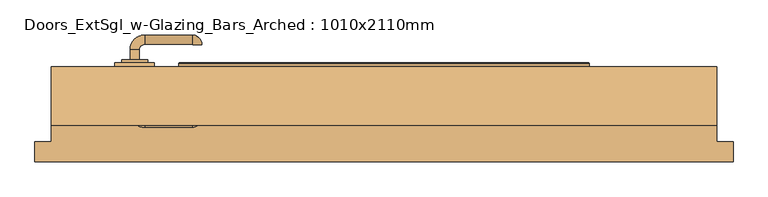
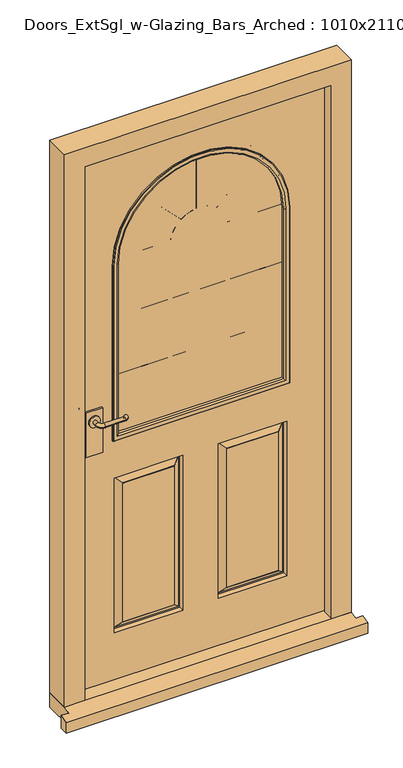
"""IFC4 building model written with IfcOpenShell, lengths in millimetres: door geometry, Doors_ExtSgl_w-Glazing_Bars_Arched : 1010x2110mm."""

from ifc_helpers import new_model, si_unit, point, frame, frame_2d, origin, place, context, project, spatial, polyline, circle_curve, ellipse_curve, trimmed, segment, composite_curve, outline, extrude, faceted_brep, source, transform, mapped, element, save
from ifc_brep_helpers import plane_surface, cylinder_surface, revolved_surface, advanced_brep


def doors_extsgl_w_glazing_bars_arched_1010x2110mm_5c897e1f(model_context):
    return source(origin(), model_context, "Body", "SolidModel", [
        extrude(outline(composite_curve([segment(trimmed(circle_curve(frame_2d((1050.0, -378.5)), 20.0), [point((1050.0, -398.5))], [point((1050.0, -358.5))], False, "CARTESIAN"), True, "CONTINUOUS"), segment(trimmed(circle_curve(frame_2d((1050.0, -378.5)), 20.0), [point((1050.0, -358.5))], [point((1050.0, -398.5))], False, "CARTESIAN"), True, "CONTINUOUS")], self_intersect=False)), frame((0.0, 18.4, 0.0), z_axis=(0.0, 1.0, 0.0), x_axis=(0.0, 0.0, 1.0)), (0.0, 0.0, 1.0), 4.5929895),
        advanced_brep(
        [(-371.5, 22.9929895, 1050.0), (-385.5, 22.9929895, 1050.0), (-371.5, 38.4, 1050.0), (-385.5, 38.4, 1050.0), (-363.5, 60.4, 1050.0), (-363.5, 46.4, 1050.0), (-291.5, 46.4, 1050.0), (-291.5, 60.4, 1050.0), (-290.5, 45.4, 1050.0), (-276.5, 45.4, 1050.0)],
        [
            (0, 1, circle_curve(frame((-378.5, 22.9929895, 1050.0), z_axis=(0.0, -1.0, 0.0), x_axis=(-1.0, 0.0, 0.0)), 7.0)),
            (1, 0, circle_curve(frame((-378.5, 22.9929895, 1050.0), z_axis=(0.0, -1.0, 0.0), x_axis=(-1.0, 0.0, 0.0)), 7.0)),
            (0, 2),
            (2, 3, circle_curve(frame((-378.5, 38.4, 1050.0), z_axis=(0.0, -1.0, 0.0), x_axis=(-1.0, 0.0, 0.0)), 7.0)),
            (3, 1),
            (3, 2, circle_curve(frame((-378.5, 38.4, 1050.0), z_axis=(0.0, -1.0, 0.0), x_axis=(-1.0, 0.0, 0.0)), 7.0)),
            (4, 3, circle_curve(frame((-363.5, 38.4, 1050.0), z_axis=(0.0, 0.0, 1.0), x_axis=(-1.0, 0.0, 0.0)), 22.0)),
            (2, 5, circle_curve(frame((-363.5, 38.4, 1050.0), z_axis=(0.0, 0.0, -1.0), x_axis=(-1.0, 0.0, 0.0)), 8.0)),
            (5, 4, circle_curve(frame((-363.5, 53.4, 1050.0), z_axis=(-1.0, 0.0, 0.0), x_axis=(0.0, 1.0, 0.0)), 7.0)),
            (4, 5, circle_curve(frame((-363.5, 53.4, 1050.0), z_axis=(-1.0, 0.0, 0.0), x_axis=(0.0, 1.0, 0.0)), 7.0)),
            (5, 6),
            (6, 7, circle_curve(frame((-291.5, 53.4, 1050.0), z_axis=(-1.0, 0.0, 0.0), x_axis=(0.0, 1.0, 0.0)), 7.0)),
            (7, 4),
            (7, 6, circle_curve(frame((-291.5, 53.4, 1050.0), z_axis=(-1.0, 0.0, 0.0), x_axis=(0.0, 1.0, 0.0)), 7.0)),
            (8, 9, circle_curve(frame((-283.5, 45.4, 1050.0), z_axis=(0.0, -1.0, 0.0), x_axis=(1.0, 0.0, 0.0)), 7.0)),
            (9, 8, circle_curve(frame((-283.5, 45.4, 1050.0), z_axis=(0.0, -1.0, 0.0), x_axis=(1.0, 0.0, 0.0)), 7.0)),
            (9, 7, circle_curve(frame((-291.5, 45.4, 1050.0), z_axis=(0.0, 0.0, 1.0), x_axis=(0.0, 1.0, 0.0)), 15.0)),
            (6, 8, circle_curve(frame((-291.5, 45.4, 1050.0), z_axis=(0.0, 0.0, -1.0), x_axis=(0.0, 1.0, 0.0)), 1.0)),
        ],
        [
            plane_surface(frame((-378.5, 22.9929895, 1050.0), z_axis=(0.0, -1.0, 0.0), x_axis=(0.0, 0.0, 1.0))),
            cylinder_surface(frame((-378.5, 22.9929895, 1050.0), z_axis=(0.0, -1.0, 0.0), x_axis=(-1.0, 0.0, 0.0)), 7.0),
            revolved_surface(trimmed(ellipse_curve(frame((-378.5, 38.4, 1050.0), z_axis=(0.0, -1.0, 0.0), x_axis=(-1.0, 0.0, 0.0)), 7.0, 7.0), [point((-371.5, 38.4, 1050.0))], [point((-385.5, 38.4, 1050.0))], True, "CARTESIAN"), (-363.5, 38.4, 1050.0), (0.0, 0.0, -1.0)),
            revolved_surface(trimmed(ellipse_curve(frame((-378.5, 38.4, 1050.0), z_axis=(0.0, -1.0, 0.0), x_axis=(-1.0, 0.0, 0.0)), 7.0, 7.0), [point((-385.5, 38.4, 1050.0))], [point((-371.5, 38.4, 1050.0))], True, "CARTESIAN"), (-363.5, 38.4, 1050.0), (0.0, 0.0, -1.0)),
            cylinder_surface(frame((-363.5, 53.4, 1050.0), z_axis=(-1.0, 0.0, 0.0), x_axis=(0.0, 1.0, 0.0)), 7.0),
            plane_surface(frame((-283.5, 45.4, 1050.0), z_axis=(0.0, -1.0, 0.0), x_axis=(0.0, 0.0, 1.0))),
            revolved_surface(trimmed(ellipse_curve(frame((-291.5, 53.4, 1050.0), z_axis=(-1.0, 0.0, 0.0), x_axis=(0.0, 1.0, 0.0)), 7.0, 7.0), [point((-291.5, 46.4, 1050.0))], [point((-291.5, 60.4, 1050.0))], True, "CARTESIAN"), (-291.5, 45.4, 1050.0), (0.0, 0.0, -1.0)),
            revolved_surface(trimmed(ellipse_curve(frame((-291.5, 53.4, 1050.0), z_axis=(-1.0, 0.0, 0.0), x_axis=(0.0, 1.0, 0.0)), 7.0, 7.0), [point((-291.5, 60.4, 1050.0))], [point((-291.5, 46.4, 1050.0))], True, "CARTESIAN"), (-291.5, 45.4, 1050.0), (0.0, 0.0, -1.0)),
        ],
        [
            (0, [[1, 2]]),
            (1, [[-1, 3, 4, 5]]),
            (1, [[-2, -5, 6, -3]]),
            (2, [[7, -4, 8, 9]]),
            (3, [[-8, -6, -7, 10]]),
            (4, [[-9, 11, 12, 13]]),
            (4, [[-10, -13, 14, -11]]),
            (5, [[15, 16]]),
            (6, [[17, -12, 18, -16]]),
            (7, [[-18, -14, -17, -15]]),
        ],
    ),
        extrude(outline(polyline([(-348.5, 12.4), (-408.5, 12.4), (-408.5, 18.4), (-348.5, 18.4), (-348.5, 12.4)])), frame((0.0, 0.0, 925.0), z_axis=(0.0, 0.0, 1.0), x_axis=(1.0, 0.0, 0.0)), (0.0, 0.0, 1.0), 165.0),
        extrude(outline(composite_curve([segment(trimmed(circle_curve(frame_2d((1050.0, -378.5)), 20.0), [point((1050.0, -398.5))], [point((1050.0, -358.5))], False, "CARTESIAN"), True, "CONTINUOUS"), segment(trimmed(circle_curve(frame_2d((1050.0, -378.5)), 20.0), [point((1050.0, -358.5))], [point((1050.0, -398.5))], False, "CARTESIAN"), True, "CONTINUOUS")], self_intersect=False)), frame((0.0, -42.1929895, 0.0), z_axis=(0.0, 1.0, 0.0), x_axis=(0.0, 0.0, 1.0)), (0.0, 0.0, 1.0), 4.5929895),
        advanced_brep(
        [(-371.5, -42.1929895, 1050.0), (-385.5, -42.1929895, 1050.0), (-385.5, -57.6, 1050.0), (-371.5, -57.6, 1050.0), (-363.5, -79.6, 1050.0), (-363.5, -65.6, 1050.0), (-291.5, -79.6, 1050.0), (-291.5, -65.6, 1050.0), (-290.5, -64.6, 1050.0), (-276.5, -64.6, 1050.0)],
        [
            (0, 1, circle_curve(frame((-378.5, -42.1929895, 1050.0), z_axis=(0.0, 1.0, 0.0), x_axis=(-1.0, 0.0, 0.0)), 7.0)),
            (1, 0, circle_curve(frame((-378.5, -42.1929895, 1050.0), z_axis=(0.0, 1.0, 0.0), x_axis=(-1.0, 0.0, 0.0)), 7.0)),
            (1, 2),
            (2, 3, circle_curve(frame((-378.5, -57.6, 1050.0), z_axis=(0.0, 1.0, 0.0), x_axis=(-1.0, 0.0, 0.0)), 7.0)),
            (3, 0),
            (3, 2, circle_curve(frame((-378.5, -57.6, 1050.0), z_axis=(0.0, 1.0, 0.0), x_axis=(-1.0, 0.0, 0.0)), 7.0)),
            (4, 5, circle_curve(frame((-363.5, -72.6, 1050.0), z_axis=(-1.0, 0.0, 0.0), x_axis=(0.0, -1.0, 0.0)), 7.0)),
            (5, 3, circle_curve(frame((-363.5, -57.6, 1050.0), z_axis=(0.0, 0.0, -1.0), x_axis=(-1.0, 0.0, 0.0)), 8.0)),
            (2, 4, circle_curve(frame((-363.5, -57.6, 1050.0), z_axis=(0.0, 0.0, 1.0), x_axis=(-1.0, 0.0, 0.0)), 22.0)),
            (5, 4, circle_curve(frame((-363.5, -72.6, 1050.0), z_axis=(-1.0, 0.0, 0.0), x_axis=(0.0, -1.0, 0.0)), 7.0)),
            (4, 6),
            (6, 7, circle_curve(frame((-291.5, -72.6, 1050.0), z_axis=(-1.0, 0.0, 0.0), x_axis=(0.0, -1.0, 0.0)), 7.0)),
            (7, 5),
            (7, 6, circle_curve(frame((-291.5, -72.6, 1050.0), z_axis=(-1.0, 0.0, 0.0), x_axis=(0.0, -1.0, 0.0)), 7.0)),
            (8, 9, circle_curve(frame((-283.5, -64.6, 1050.0), z_axis=(0.0, 1.0, 0.0), x_axis=(1.0, 0.0, 0.0)), 7.0)),
            (9, 8, circle_curve(frame((-283.5, -64.6, 1050.0), z_axis=(0.0, 1.0, 0.0), x_axis=(1.0, 0.0, 0.0)), 7.0)),
            (8, 7, circle_curve(frame((-291.5, -64.6, 1050.0), z_axis=(0.0, 0.0, -1.0), x_axis=(0.0, -1.0, 0.0)), 1.0)),
            (6, 9, circle_curve(frame((-291.5, -64.6, 1050.0), z_axis=(0.0, 0.0, 1.0), x_axis=(0.0, -1.0, 0.0)), 15.0)),
        ],
        [
            plane_surface(frame((-378.5, -42.1929895, 1050.0), z_axis=(0.0, 1.0, 0.0), x_axis=(0.0, 0.0, 1.0))),
            cylinder_surface(frame((-378.5, -42.1929895, 1050.0), z_axis=(0.0, 1.0, 0.0), x_axis=(-1.0, 0.0, 0.0)), 7.0),
            revolved_surface(trimmed(ellipse_curve(frame((-378.5, -57.6, 1050.0), z_axis=(0.0, -1.0, 0.0), x_axis=(-1.0, 0.0, 0.0)), 7.0, 7.0), [point((-371.5, -57.6, 1050.0))], [point((-385.5, -57.6, 1050.0))], True, "CARTESIAN"), (-363.5, -57.6, 1050.0), (0.0, 0.0, -1.0)),
            revolved_surface(trimmed(ellipse_curve(frame((-378.5, -57.6, 1050.0), z_axis=(0.0, -1.0, 0.0), x_axis=(-1.0, 0.0, 0.0)), 7.0, 7.0), [point((-385.5, -57.6, 1050.0))], [point((-371.5, -57.6, 1050.0))], True, "CARTESIAN"), (-363.5, -57.6, 1050.0), (0.0, 0.0, -1.0)),
            cylinder_surface(frame((-363.5, -72.6, 1050.0), z_axis=(-1.0, 0.0, 0.0), x_axis=(0.0, -1.0, 0.0)), 7.0),
            plane_surface(frame((-283.5, -64.6, 1050.0), z_axis=(0.0, 1.0, 0.0), x_axis=(0.0, 0.0, 1.0))),
            revolved_surface(trimmed(ellipse_curve(frame((-291.5, -72.6, 1050.0), z_axis=(1.0, 0.0, 0.0), x_axis=(0.0, -1.0, 0.0)), 7.0, 7.0), [point((-291.5, -65.6, 1050.0))], [point((-291.5, -79.6, 1050.0))], True, "CARTESIAN"), (-291.5, -64.6, 1050.0), (0.0, 0.0, -1.0)),
            revolved_surface(trimmed(ellipse_curve(frame((-291.5, -72.6, 1050.0), z_axis=(1.0, 0.0, 0.0), x_axis=(0.0, -1.0, 0.0)), 7.0, 7.0), [point((-291.5, -79.6, 1050.0))], [point((-291.5, -65.6, 1050.0))], True, "CARTESIAN"), (-291.5, -64.6, 1050.0), (0.0, 0.0, -1.0)),
        ],
        [
            (0, [[1, 2]]),
            (1, [[3, 4, 5, -2]]),
            (1, [[-5, 6, -3, -1]]),
            (2, [[7, 8, -4, 9]]),
            (3, [[10, -9, -6, -8]]),
            (4, [[11, 12, 13, -7]]),
            (4, [[-13, 14, -11, -10]]),
            (5, [[15, 16]]),
            (6, [[-15, 17, -12, 18]]),
            (7, [[-16, -18, -14, -17]]),
        ],
    ),
        extrude(outline(polyline([(-348.5, -31.6), (-348.5, -37.6), (-408.5, -37.6), (-408.5, -31.6), (-348.5, -31.6)])), frame((0.0, 0.0, 925.0), z_axis=(0.0, 0.0, 1.0), x_axis=(1.0, 0.0, 0.0)), (0.0, 0.0, 1.0), 165.0),
        faceted_brep([(434.5, -76.6, 54.5), (434.5, -34.6, 54.5), (456.5, -34.6, 54.5), (456.5, 12.4, 54.5), (505.0, 12.4, 54.5), (505.0, -76.6, 54.5), (505.0, -76.6, 2110.0), (-505.0, -76.6, 2110.0), (-505.0, -76.6, 54.5), (-434.5, -76.6, 54.5), (-434.5, -76.6, 2039.5), (434.5, -76.6, 2039.5), (505.0, 12.4, 2110.0), (456.5, 12.4, 2061.5), (-456.5, 12.4, 2061.5), (-456.5, 12.4, 54.5), (-505.0, 12.4, 54.5), (-505.0, 12.4, 2110.0), (456.5, -34.6, 2061.5), (434.5, -34.6, 2039.5), (-434.5, -34.6, 2039.5), (-434.5, -34.6, 54.5), (-456.5, -34.6, 54.5), (-456.5, -34.6, 2061.5)], [[[0, 1, 2, 3, 4, 5]], [[5, 6, 7, 8, 9, 10, 11, 0]], [[4, 12, 6, 5]], [[3, 13, 14, 15, 16, 17, 12, 4]], [[2, 18, 13, 3]], [[1, 19, 20, 21, 22, 23, 18, 2]], [[0, 11, 19, 1]], [[9, 21, 20, 10]], [[8, 16, 15, 22, 21, 9]], [[7, 17, 16, 8]], [[14, 23, 22, 15]], [[6, 12, 17, 7]], [[13, 18, 23, 14]], [[10, 20, 19, 11]]]),
        advanced_brep(
        [(453.5, 12.4, 58.5), (-454.4250294, 12.4, 58.5), (-454.4250294, 12.4, 2058.5), (453.5, 12.4, 2058.5), (-303.5, 12.4, 958.5), (303.5, 12.4, 958.5), (303.5, 12.4, 1605.0), (-303.5, 12.4, 1605.0), (-62.5, 12.4, 808.5), (-303.5, 12.4, 808.5), (-303.5, 12.4, 233.5), (-62.5, 12.4, 233.5), (303.5, 12.4, 808.5), (62.5, 12.4, 808.5), (62.5, 12.4, 233.5), (303.5, 12.4, 233.5), (-92.5, 12.4, 263.5), (-273.5, 12.4, 263.5), (-273.5, 12.4, 778.5), (-92.5, 12.4, 778.5), (273.5, 12.4, 263.5), (92.5, 12.4, 263.5), (92.5, 12.4, 778.5), (273.5, 12.4, 778.5), (453.5, -31.6, 58.5), (453.5, -31.6, 2058.5), (-454.4250294, -31.6, 2058.5), (-454.4250294, -31.6, 58.5), (-303.5, -31.6, 958.5), (-303.5, -31.6, 1605.0), (303.5, -31.6, 1605.0), (303.5, -31.6, 958.5), (62.5, -31.6, 808.5), (303.5, -31.6, 808.5), (303.5, -31.6, 233.5), (62.5, -31.6, 233.5), (-303.5, -31.6, 808.5), (-62.5, -31.6, 808.5), (-62.5, -31.6, 233.5), (-303.5, -31.6, 233.5), (92.5, -31.6, 263.5), (273.5, -31.6, 263.5), (273.5, -31.6, 778.5), (92.5, -31.6, 778.5), (-273.5, -31.6, 263.5), (-92.5, -31.6, 263.5), (-92.5, -31.6, 778.5), (-273.5, -31.6, 778.5), (65.5, -16.6, 805.5), (65.5, -16.6, 236.5), (90.5, -30.6, 780.5), (70.5, -16.6, 800.5), (70.5, -16.6, 241.5), (90.5, -30.6, 261.5), (92.5, -30.6, 778.5), (92.5, -30.6, 263.5), (300.5, -16.6, 236.5), (295.5, -16.6, 241.5), (275.5, -30.6, 261.5), (273.5, -30.6, 263.5), (300.5, -16.6, 805.5), (295.5, -16.6, 800.5), (275.5, -30.6, 780.5), (273.5, -30.6, 778.5), (-300.5, -16.6, 805.5), (-300.5, -16.6, 236.5), (-275.5, -30.6, 780.5), (-295.5, -16.6, 800.5), (-295.5, -16.6, 241.5), (-275.5, -30.6, 261.5), (-273.5, -30.6, 778.5), (-273.5, -30.6, 263.5), (-65.5, -16.6, 236.5), (-70.5, -16.6, 241.5), (-90.5, -30.6, 261.5), (-92.5, -30.6, 263.5), (-65.5, -16.6, 805.5), (-70.5, -16.6, 800.5), (-90.5, -30.6, 780.5), (-92.5, -30.6, 778.5), (-92.5, 11.4, 263.5), (-92.5, 11.4, 778.5), (-70.5, -2.6, 241.5), (-90.5, 11.4, 261.5), (-90.5, 11.4, 780.5), (-70.5, -2.6, 800.5), (-65.5, -2.6, 236.5), (-65.5, -2.6, 805.5), (-273.5, 11.4, 778.5), (-275.5, 11.4, 780.5), (-295.5, -2.6, 800.5), (-300.5, -2.6, 805.5), (-273.5, 11.4, 263.5), (-275.5, 11.4, 261.5), (-295.5, -2.6, 241.5), (-300.5, -2.6, 236.5), (300.5, -2.6, 805.5), (300.5, -2.6, 236.5), (275.5, 11.4, 780.5), (295.5, -2.6, 800.5), (295.5, -2.6, 241.5), (275.5, 11.4, 261.5), (273.5, 11.4, 778.5), (273.5, 11.4, 263.5), (65.5, -2.6, 236.5), (70.5, -2.6, 241.5), (90.5, 11.4, 261.5), (92.5, 11.4, 263.5), (65.5, -2.6, 805.5), (70.5, -2.6, 800.5), (90.5, 11.4, 780.5), (92.5, 11.4, 778.5)],
        [
            (0, 1),
            (1, 2),
            (2, 3),
            (3, 0),
            (4, 5),
            (5, 6),
            (6, 7, circle_curve(frame((0.0, 12.4, 1605.0), z_axis=(0.0, -1.0, 0.0), x_axis=(1.0, 0.0, 0.0)), 303.5)),
            (7, 4),
            (8, 9),
            (9, 10),
            (10, 11),
            (11, 8),
            (12, 13),
            (13, 14),
            (14, 15),
            (15, 12),
            (16, 17),
            (17, 18),
            (18, 19),
            (19, 16),
            (20, 21),
            (21, 22),
            (22, 23),
            (23, 20),
            (24, 25),
            (25, 26),
            (26, 27),
            (27, 24),
            (28, 29),
            (29, 30, circle_curve(frame((0.0, -31.6, 1605.0), z_axis=(0.0, 1.0, 0.0), x_axis=(1.0, 0.0, 0.0)), 303.5)),
            (30, 31),
            (31, 28),
            (32, 33),
            (33, 34),
            (34, 35),
            (35, 32),
            (36, 37),
            (37, 38),
            (38, 39),
            (39, 36),
            (40, 41),
            (41, 42),
            (42, 43),
            (43, 40),
            (44, 45),
            (45, 46),
            (46, 47),
            (47, 44),
            (3, 25),
            (24, 0),
            (2, 26),
            (1, 27),
            (7, 29),
            (28, 4),
            (6, 30),
            (5, 31),
            (48, 32),
            (35, 49),
            (49, 48),
            (50, 51),
            (51, 52),
            (52, 53),
            (53, 50),
            (43, 54),
            (54, 55),
            (55, 40),
            (34, 56),
            (56, 49),
            (52, 57),
            (57, 58),
            (58, 53),
            (55, 59),
            (59, 41),
            (33, 60),
            (60, 56),
            (57, 61),
            (61, 62),
            (62, 58),
            (59, 63),
            (63, 42),
            (48, 60),
            (51, 61),
            (50, 62),
            (54, 63),
            (64, 36),
            (39, 65),
            (65, 64),
            (66, 67),
            (67, 68),
            (68, 69),
            (69, 66),
            (47, 70),
            (70, 71),
            (71, 44),
            (38, 72),
            (72, 65),
            (68, 73),
            (73, 74),
            (74, 69),
            (71, 75),
            (75, 45),
            (37, 76),
            (76, 72),
            (73, 77),
            (77, 78),
            (78, 74),
            (75, 79),
            (79, 46),
            (64, 76),
            (67, 77),
            (66, 78),
            (70, 79),
            (80, 16),
            (19, 81),
            (81, 80),
            (82, 83),
            (83, 84),
            (84, 85),
            (85, 82),
            (11, 86),
            (86, 87),
            (87, 8),
            (18, 88),
            (88, 81),
            (84, 89),
            (89, 90),
            (90, 85),
            (87, 91),
            (91, 9),
            (17, 92),
            (92, 88),
            (89, 93),
            (93, 94),
            (94, 90),
            (91, 95),
            (95, 10),
            (80, 92),
            (83, 93),
            (82, 94),
            (86, 95),
            (96, 12),
            (15, 97),
            (97, 96),
            (98, 99),
            (99, 100),
            (100, 101),
            (101, 98),
            (23, 102),
            (102, 103),
            (103, 20),
            (14, 104),
            (104, 97),
            (100, 105),
            (105, 106),
            (106, 101),
            (103, 107),
            (107, 21),
            (13, 108),
            (108, 104),
            (105, 109),
            (109, 110),
            (110, 106),
            (107, 111),
            (111, 22),
            (96, 108),
            (99, 109),
            (98, 110),
            (102, 111),
        ],
        [
            plane_surface(frame((453.5, 12.4, 58.5), z_axis=(0.0, 1.0, 0.0), x_axis=(0.0, 0.0, 1.0))),
            plane_surface(frame((453.5, -31.6, 58.5), z_axis=(0.0, -1.0, 0.0), x_axis=(0.0, 0.0, -1.0))),
            plane_surface(frame((453.5, 12.4, 58.5), z_axis=(1.0, 0.0, 0.0), x_axis=(0.0, -1.0, 0.0))),
            plane_surface(frame((453.5, 12.4, 2058.5), z_axis=(0.0, 0.0, 1.0), x_axis=(0.0, -1.0, 0.0))),
            plane_surface(frame((-454.4250294, 12.4, 2058.5), z_axis=(-1.0, 0.0, 0.0), x_axis=(0.0, -1.0, 0.0))),
            plane_surface(frame((-454.4250294, 12.4, 58.5), z_axis=(0.0, 0.0, -1.0), x_axis=(0.0, -1.0, 0.0))),
            plane_surface(frame((-303.5, 12.4, 958.5), z_axis=(1.0, 0.0, 0.0), x_axis=(0.0, -1.0, 0.0))),
            revolved_surface(polyline([(303.5, -31.6, 1605.0), (303.5, 12.4, 1605.0)]), (0.0, 12.4, 1605.0), (0.0, -1.0, 0.0)),
            plane_surface(frame((303.5, 12.4, 1605.0), z_axis=(-1.0, 0.0, 0.0), x_axis=(0.0, -1.0, 0.0))),
            plane_surface(frame((303.5, 12.4, 958.5), z_axis=(0.0, 0.0, 1.0), x_axis=(0.0, -1.0, 0.0))),
            plane_surface(frame((62.5, -31.6, 808.5), z_axis=(0.9805806756909202, -0.19611613513818407, 0.0), x_axis=(0.0, 0.0, -1.0))),
            plane_surface(frame((70.5, -16.6, 800.5), z_axis=(-0.5734623443633278, -0.8192319205190408, 0.0), x_axis=(0.0, 0.0, -1.0))),
            plane_surface(frame((92.5, -30.6, 778.5), z_axis=(-1.0, 0.0, 0.0), x_axis=(0.0, 0.0, -1.0))),
            plane_surface(frame((62.5, -31.6, 233.5), z_axis=(0.0, -0.19611613513818726, 0.9805806756909196), x_axis=(1.0, 0.0, 0.0))),
            plane_surface(frame((70.5, -16.6, 241.5), z_axis=(0.0, -0.819231920519039, -0.5734623443633305), x_axis=(1.0, 0.0, 0.0))),
            plane_surface(frame((92.5, -30.6, 263.5), z_axis=(0.0, 0.0, -1.0), x_axis=(1.0, 0.0, 0.0))),
            plane_surface(frame((303.5, -31.6, 233.5), z_axis=(-0.9805806756909189, -0.19611613513819046, 0.0), x_axis=(0.0, 0.0, 1.0))),
            plane_surface(frame((295.5, -16.6, 241.5), z_axis=(0.5734623443633332, -0.8192319205190371, 0.0), x_axis=(0.0, 0.0, 1.0))),
            plane_surface(frame((273.5, -30.6, 263.5), z_axis=(1.0, 0.0, 0.0), x_axis=(0.0, 0.0, 1.0))),
            plane_surface(frame((303.5, -31.6, 808.5), z_axis=(0.0, -0.19611613513818726, -0.9805806756909196), x_axis=(-1.0, 0.0, 0.0))),
            plane_surface(frame((300.5, -16.6, 805.5), z_axis=(0.0, -1.0, 0.0), x_axis=(-1.0, 0.0, 0.0))),
            plane_surface(frame((295.5, -16.6, 800.5), z_axis=(0.0, -0.819231920519039, 0.5734623443633305), x_axis=(-1.0, 0.0, 0.0))),
            plane_surface(frame((275.5, -30.6, 780.5), z_axis=(0.0, -1.0, 0.0), x_axis=(-1.0, 0.0, 0.0))),
            plane_surface(frame((273.5, -30.6, 778.5), z_axis=(0.0, 0.0, 1.0), x_axis=(-1.0, 0.0, 0.0))),
            plane_surface(frame((-303.5, -31.6, 808.5), z_axis=(0.9805806756909202, -0.19611613513818407, 0.0), x_axis=(0.0, 0.0, -1.0))),
            plane_surface(frame((-295.5, -16.6, 800.5), z_axis=(-0.5734623443633278, -0.8192319205190408, 0.0), x_axis=(0.0, 0.0, -1.0))),
            plane_surface(frame((-273.5, -30.6, 778.5), z_axis=(-1.0, 0.0, 0.0), x_axis=(0.0, 0.0, -1.0))),
            plane_surface(frame((-303.5, -31.6, 233.5), z_axis=(0.0, -0.19611613513818724, 0.9805806756909196), x_axis=(1.0, 0.0, 0.0))),
            plane_surface(frame((-295.5, -16.6, 241.5), z_axis=(0.0, -0.819231920519039, -0.5734623443633305), x_axis=(1.0, 0.0, 0.0))),
            plane_surface(frame((-273.5, -30.6, 263.5), z_axis=(0.0, 0.0, -1.0), x_axis=(1.0, 0.0, 0.0))),
            plane_surface(frame((-62.5, -31.6, 233.5), z_axis=(-0.9805806756909189, -0.1961161351381904, 0.0), x_axis=(0.0, 0.0, 1.0))),
            plane_surface(frame((-70.5, -16.6, 241.5), z_axis=(0.5734623443633332, -0.8192319205190371, 0.0), x_axis=(0.0, 0.0, 1.0))),
            plane_surface(frame((-92.5, -30.6, 263.5), z_axis=(1.0, 0.0, 0.0), x_axis=(0.0, 0.0, 1.0))),
            plane_surface(frame((-62.5, -31.6, 808.5), z_axis=(0.0, -0.19611613513818724, -0.9805806756909196), x_axis=(-1.0, 0.0, 0.0))),
            plane_surface(frame((-65.5, -16.6, 805.5), z_axis=(0.0, -1.0, 0.0), x_axis=(-1.0, 0.0, 0.0))),
            plane_surface(frame((-70.5, -16.6, 800.5), z_axis=(0.0, -0.819231920519039, 0.5734623443633305), x_axis=(-1.0, 0.0, 0.0))),
            plane_surface(frame((-90.5, -30.6, 780.5), z_axis=(0.0, -1.0, 0.0), x_axis=(-1.0, 0.0, 0.0))),
            plane_surface(frame((-92.5, -30.6, 778.5), z_axis=(0.0, 0.0, 1.0), x_axis=(-1.0, 0.0, 0.0))),
            plane_surface(frame((-92.5, 12.4, 263.5), z_axis=(1.0, 0.0, 0.0), x_axis=(0.0, 0.0, 1.0))),
            plane_surface(frame((-90.5, 11.4, 261.5), z_axis=(0.5734623443633224, 0.8192319205190447, 0.0), x_axis=(0.0, 0.0, 1.0))),
            plane_surface(frame((-65.5, -2.6, 236.5), z_axis=(-0.9805806756909214, 0.1961161351381778, 0.0), x_axis=(0.0, 0.0, 1.0))),
            plane_surface(frame((-92.5, 12.4, 778.5), z_axis=(0.0, 0.0, 1.0), x_axis=(-1.0, 0.0, 0.0))),
            plane_surface(frame((-90.5, 11.4, 780.5), z_axis=(0.0, 0.8192319205190428, 0.5734623443633251), x_axis=(-1.0, 0.0, 0.0))),
            plane_surface(frame((-65.5, -2.6, 805.5), z_axis=(0.0, 0.19611613513818096, -0.9805806756909208), x_axis=(-1.0, 0.0, 0.0))),
            plane_surface(frame((-273.5, 12.4, 778.5), z_axis=(-1.0, 0.0, 0.0), x_axis=(0.0, 0.0, -1.0))),
            plane_surface(frame((-275.5, 11.4, 780.5), z_axis=(-0.5734623443633277, 0.8192319205190409, 0.0), x_axis=(0.0, 0.0, -1.0))),
            plane_surface(frame((-300.5, -2.6, 805.5), z_axis=(0.9805806756909201, 0.19611613513818418, 0.0), x_axis=(0.0, 0.0, -1.0))),
            plane_surface(frame((-273.5, 12.4, 263.5), z_axis=(0.0, 0.0, -1.0), x_axis=(1.0, 0.0, 0.0))),
            plane_surface(frame((-273.5, 11.4, 263.5), z_axis=(0.0, 1.0, 0.0), x_axis=(1.0, 0.0, 0.0))),
            plane_surface(frame((-275.5, 11.4, 261.5), z_axis=(0.0, 0.8192319205190429, -0.573462344363325), x_axis=(1.0, 0.0, 0.0))),
            plane_surface(frame((-295.5, -2.6, 241.5), z_axis=(0.0, 1.0, 0.0), x_axis=(1.0, 0.0, 0.0))),
            plane_surface(frame((-300.5, -2.6, 236.5), z_axis=(0.0, 0.19611613513818107, 0.9805806756909208), x_axis=(1.0, 0.0, 0.0))),
            plane_surface(frame((303.5, 12.4, 808.5), z_axis=(-0.9805806756909202, 0.19611613513818407, 0.0), x_axis=(0.0, 0.0, -1.0))),
            plane_surface(frame((295.5, -2.6, 800.5), z_axis=(0.5734623443633278, 0.8192319205190408, 0.0), x_axis=(0.0, 0.0, -1.0))),
            plane_surface(frame((273.5, 11.4, 778.5), z_axis=(1.0, 0.0, 0.0), x_axis=(0.0, 0.0, -1.0))),
            plane_surface(frame((303.5, 12.4, 233.5), z_axis=(0.0, 0.19611613513818724, 0.9805806756909196), x_axis=(-1.0, 0.0, 0.0))),
            plane_surface(frame((295.5, -2.6, 241.5), z_axis=(0.0, 0.819231920519039, -0.5734623443633305), x_axis=(-1.0, 0.0, 0.0))),
            plane_surface(frame((273.5, 11.4, 263.5), z_axis=(0.0, 0.0, -1.0), x_axis=(-1.0, 0.0, 0.0))),
            plane_surface(frame((62.5, 12.4, 233.5), z_axis=(0.9805806756909189, 0.19611613513819046, 0.0), x_axis=(0.0, 0.0, 1.0))),
            plane_surface(frame((70.5, -2.6, 241.5), z_axis=(-0.5734623443633331, 0.8192319205190371, 0.0), x_axis=(0.0, 0.0, 1.0))),
            plane_surface(frame((92.5, 11.4, 263.5), z_axis=(-1.0, 0.0, 0.0), x_axis=(0.0, 0.0, 1.0))),
            plane_surface(frame((62.5, 12.4, 808.5), z_axis=(0.0, 0.19611613513818735, -0.9805806756909196), x_axis=(1.0, 0.0, 0.0))),
            plane_surface(frame((65.5, -2.6, 805.5), z_axis=(0.0, 1.0, 0.0), x_axis=(1.0, 0.0, 0.0))),
            plane_surface(frame((70.5, -2.6, 800.5), z_axis=(0.0, 0.819231920519039, 0.5734623443633303), x_axis=(1.0, 0.0, 0.0))),
            plane_surface(frame((90.5, 11.4, 780.5), z_axis=(0.0, 1.0, 0.0), x_axis=(1.0, 0.0, 0.0))),
            plane_surface(frame((92.5, 11.4, 778.5), z_axis=(0.0, 0.0, 1.0), x_axis=(1.0, 0.0, 0.0))),
        ],
        [
            (0, [[1, 2, 3, 4], [5, 6, 7, 8], [9, 10, 11, 12], [13, 14, 15, 16]]),
            (0, [[17, 18, 19, 20]]),
            (0, [[21, 22, 23, 24]]),
            (1, [[25, 26, 27, 28], [29, 30, 31, 32], [33, 34, 35, 36], [37, 38, 39, 40]]),
            (1, [[41, 42, 43, 44]]),
            (1, [[45, 46, 47, 48]]),
            (2, [[49, -25, 50, -4]]),
            (3, [[51, -26, -49, -3]]),
            (4, [[52, -27, -51, -2]]),
            (5, [[-50, -28, -52, -1]]),
            (6, [[53, -29, 54, -8]]),
            (7, [[55, -30, -53, -7]]),
            (8, [[56, -31, -55, -6]]),
            (9, [[-54, -32, -56, -5]]),
            (10, [[57, -36, 58, 59]]),
            (11, [[60, 61, 62, 63]]),
            (12, [[-44, 64, 65, 66]]),
            (13, [[-35, 67, 68, -58]]),
            (14, [[69, 70, 71, -62]]),
            (15, [[72, 73, -41, -66]]),
            (16, [[-34, 74, 75, -67]]),
            (17, [[76, 77, 78, -70]]),
            (18, [[79, 80, -42, -73]]),
            (19, [[81, -74, -33, -57]]),
            (20, [[-68, -75, -81, -59], [82, -76, -69, -61]]),
            (21, [[83, -77, -82, -60]]),
            (22, [[-71, -78, -83, -63], [84, -79, -72, -65]]),
            (23, [[-43, -80, -84, -64]]),
            (24, [[85, -40, 86, 87]]),
            (25, [[88, 89, 90, 91]]),
            (26, [[-48, 92, 93, 94]]),
            (27, [[-39, 95, 96, -86]]),
            (28, [[97, 98, 99, -90]]),
            (29, [[100, 101, -45, -94]]),
            (30, [[-38, 102, 103, -95]]),
            (31, [[104, 105, 106, -98]]),
            (32, [[107, 108, -46, -101]]),
            (33, [[109, -102, -37, -85]]),
            (34, [[-96, -103, -109, -87], [110, -104, -97, -89]]),
            (35, [[111, -105, -110, -88]]),
            (36, [[-99, -106, -111, -91], [112, -107, -100, -93]]),
            (37, [[-47, -108, -112, -92]]),
            (38, [[113, -20, 114, 115]]),
            (39, [[116, 117, 118, 119]]),
            (40, [[-12, 120, 121, 122]]),
            (41, [[-19, 123, 124, -114]]),
            (42, [[125, 126, 127, -118]]),
            (43, [[128, 129, -9, -122]]),
            (44, [[-18, 130, 131, -123]]),
            (45, [[132, 133, 134, -126]]),
            (46, [[135, 136, -10, -129]]),
            (47, [[137, -130, -17, -113]]),
            (48, [[138, -132, -125, -117], [-124, -131, -137, -115]]),
            (49, [[139, -133, -138, -116]]),
            (50, [[140, -135, -128, -121], [-127, -134, -139, -119]]),
            (51, [[-11, -136, -140, -120]]),
            (52, [[141, -16, 142, 143]]),
            (53, [[144, 145, 146, 147]]),
            (54, [[-24, 148, 149, 150]]),
            (55, [[-15, 151, 152, -142]]),
            (56, [[153, 154, 155, -146]]),
            (57, [[156, 157, -21, -150]]),
            (58, [[-14, 158, 159, -151]]),
            (59, [[160, 161, 162, -154]]),
            (60, [[163, 164, -22, -157]]),
            (61, [[165, -158, -13, -141]]),
            (62, [[-152, -159, -165, -143], [166, -160, -153, -145]]),
            (63, [[167, -161, -166, -144]]),
            (64, [[-155, -162, -167, -147], [168, -163, -156, -149]]),
            (65, [[-23, -164, -168, -148]]),
        ],
    ),
        faceted_brep([(530.0, -131.6, 0.0), (530.0, -101.6, 0.0), (530.0, -101.6, 47.2703282), (530.0, -131.6, 38.5947221), (-530.0, -131.6, 38.5947221), (-530.0, -101.6, 47.2703282), (-530.0, -101.6, 0.0), (-530.0, -131.6, 0.0), (-505.0, -101.6, 0.0), (-505.0, 12.4, 0.0), (505.0, 12.4, 0.0), (505.0, -101.6, 0.0), (505.0, -101.6, 47.2703282), (505.0, -76.6, 54.5), (-505.0, -76.6, 54.5), (-505.0, -101.6, 47.2703282), (505.0, 12.4, 54.5), (-505.0, 12.4, 54.5)], [[[0, 1, 2, 3]], [[4, 5, 6, 7]], [[7, 6, 8, 9, 10, 11, 1, 0]], [[3, 4, 7, 0]], [[3, 2, 12, 13, 14, 15, 5, 4]], [[14, 13, 16, 17]], [[17, 16, 10, 9]], [[15, 14, 17, 9, 8]], [[8, 6, 5, 15]], [[11, 10, 16, 13, 12]], [[12, 2, 1, 11]]]),
        extrude(outline(composite_curve([segment(polyline([(958.5, -303.5), (958.5, 303.5), (1605.0, 303.5)]), True, "CONTINUOUS"), segment(trimmed(circle_curve(frame_2d((1605.0, 0.0)), 303.5), [point((1605.0, 303.5))], [point((1605.0, -303.5))], False, "CARTESIAN"), True, "CONTINUOUS"), segment(polyline([(1605.0, -303.5), (958.5, -303.5)]), True, "CONTINUOUS")], self_intersect=False)), frame((0.0, -21.6, 0.0), z_axis=(0.0, 1.0, 0.0), x_axis=(0.0, 0.0, 1.0)), (0.0, 0.0, 1.0), 24.0),
        advanced_brep(
        [(-311.5, -35.6, 950.5), (-311.5, -35.6, 1605.0), (-311.5, -31.6, 1605.0), (-311.5, -31.6, 950.5), (-309.5, -37.6, 952.5), (-309.5, -37.6, 1605.0), (-291.5, -32.6, 970.5), (-291.5, -32.6, 1605.0), (-296.5, -37.6, 1605.0), (-296.5, -37.6, 965.5), (-291.5, -21.6, 970.5), (-291.5, -21.6, 1605.0), (-303.5, -31.6, 958.5), (-303.5, -31.6, 1605.0), (-303.5, -21.6, 1605.0), (-303.5, -21.6, 958.5), (311.5, -35.6, 1605.0), (311.5, -31.6, 1605.0), (309.5, -37.6, 1605.0), (309.5, -37.6, 952.5), (296.5, -37.6, 1605.0), (296.5, -37.6, 965.5), (291.5, -32.6, 1605.0), (291.5, -21.6, 1605.0), (303.5, -21.6, 1605.0), (303.5, -21.6, 958.5), (291.5, -21.6, 970.5), (303.5, -31.6, 1605.0), (311.5, -31.6, 950.5), (303.5, -31.6, 958.5), (311.5, -35.6, 950.5), (291.5, -32.6, 970.5)],
        [
            (0, 1),
            (1, 2),
            (2, 3),
            (3, 0),
            (4, 5),
            (5, 1, circle_curve(frame((-309.5, -35.6, 1605.0), z_axis=(0.0, 0.0, -1.0), x_axis=(-1.0, 0.0, 0.0)), 2.0)),
            (0, 4, ellipse_curve(frame((-309.5, -35.6, 952.5), z_axis=(-0.7071067811865475, 0.0, 0.7071067811865475), x_axis=(-0.7071067811865472, 0.0, -0.7071067811865477)), 2.8284271, 2.0)),
            (6, 7),
            (7, 8, circle_curve(frame((-296.5, -32.6, 1605.0), z_axis=(0.0, 0.0, -1.0), x_axis=(-1.0, 0.0, 0.0)), 5.0)),
            (8, 9),
            (9, 6, ellipse_curve(frame((-296.5, -32.6, 965.5), z_axis=(-0.7071067811865475, 0.0, 0.7071067811865475), x_axis=(-0.7071067811865472, 0.0, -0.7071067811865477)), 7.0710678, 5.0)),
            (10, 11),
            (11, 7),
            (6, 10),
            (12, 13),
            (13, 14),
            (14, 15),
            (15, 12),
            (16, 17),
            (17, 2, circle_curve(frame((0.0, -31.6, 1605.0), z_axis=(0.0, -1.0, 0.0), x_axis=(-1.0, 0.0, 0.0)), 311.5)),
            (1, 16, circle_curve(frame((0.0, -35.6, 1605.0), z_axis=(0.0, 1.0, 0.0), x_axis=(-1.0, 0.0, 0.0)), 311.5)),
            (18, 16, circle_curve(frame((309.5, -35.6, 1605.0), z_axis=(0.0, 0.0, 1.0), x_axis=(1.0, 0.0, 0.0)), 2.0)),
            (5, 18, circle_curve(frame((0.0, -37.6, 1605.0), z_axis=(0.0, 1.0, 0.0), x_axis=(-1.0, 0.0, 0.0)), 309.5)),
            (4, 19),
            (19, 18),
            (20, 21),
            (21, 9),
            (8, 20, circle_curve(frame((0.0, -37.6, 1605.0), z_axis=(0.0, 1.0, 0.0), x_axis=(-1.0, 0.0, 0.0)), 296.5)),
            (22, 20, circle_curve(frame((296.5, -32.6, 1605.0), z_axis=(0.0, 0.0, 1.0), x_axis=(1.0, 0.0, 0.0)), 5.0)),
            (7, 22, circle_curve(frame((0.0, -32.6, 1605.0), z_axis=(0.0, 1.0, 0.0), x_axis=(-1.0, 0.0, 0.0)), 291.5)),
            (23, 22),
            (11, 23, circle_curve(frame((0.0, -21.6, 1605.0), z_axis=(0.0, 1.0, 0.0), x_axis=(-1.0, 0.0, 0.0)), 291.5)),
            (24, 25),
            (25, 15),
            (14, 24, circle_curve(frame((0.0, -21.6, 1605.0), z_axis=(0.0, 1.0, 0.0), x_axis=(-1.0, 0.0, 0.0)), 303.5)),
            (10, 26),
            (26, 23),
            (27, 24),
            (13, 27, circle_curve(frame((0.0, -31.6, 1605.0), z_axis=(0.0, 1.0, 0.0), x_axis=(-1.0, 0.0, 0.0)), 303.5)),
            (17, 28),
            (28, 3),
            (12, 29),
            (29, 27),
            (16, 30),
            (30, 28),
            (19, 30, ellipse_curve(frame((309.5, -35.6, 952.5), z_axis=(0.7071067811865475, 0.0, 0.7071067811865475), x_axis=(-0.7071067811865475, 0.0, 0.7071067811865476)), 2.8284271, 2.0)),
            (22, 31),
            (31, 21, ellipse_curve(frame((296.5, -32.6, 965.5), z_axis=(0.7071067811865475, 0.0, 0.7071067811865475), x_axis=(-0.7071067811865475, 0.0, 0.7071067811865476)), 7.0710678, 5.0)),
            (26, 31),
            (29, 25),
            (30, 0),
            (31, 6),
        ],
        [
            plane_surface(frame((-311.5, -31.6, 950.5), z_axis=(-1.0, 0.0, 0.0), x_axis=(0.0, 0.0, 1.0))),
            cylinder_surface(frame((-309.5, -35.6, 958.5), z_axis=(0.0, 0.0, -1.0), x_axis=(-1.0, 0.0, 0.0)), 2.0),
            cylinder_surface(frame((-296.5, -32.6, 958.5), z_axis=(0.0, 0.0, -1.0), x_axis=(-1.0, 0.0, 0.0)), 5.0),
            plane_surface(frame((-291.5, -32.6, 970.5), z_axis=(1.0, 0.0, 0.0), x_axis=(0.0, 0.0, 1.0))),
            plane_surface(frame((-303.5, -21.6, 958.5), z_axis=(-1.0, 0.0, 0.0), x_axis=(0.0, 0.0, 1.0))),
            cylinder_surface(frame((0.0, -31.6, 1605.0), z_axis=(0.0, -1.0, 0.0), x_axis=(-1.0, 0.0, 0.0)), 311.5),
            revolved_surface(trimmed(ellipse_curve(frame((-309.5, -35.6, 1605.0), z_axis=(0.0, 0.0, 1.0), x_axis=(-1.0, 0.0, 0.0)), 2.0, 2.0), [point((-311.5, -35.6, 1605.0))], [point((-309.5, -37.6, 1605.0))], True, "CARTESIAN"), (0.0, -31.6, 1605.0), (0.0, -1.0, 0.0)),
            plane_surface(frame((0.0, -37.6, 1605.0), z_axis=(0.0, -1.0, 0.0), x_axis=(-1.0, 0.0, 0.0))),
            revolved_surface(trimmed(ellipse_curve(frame((-296.5, -32.6, 1605.0), z_axis=(0.0, 0.0, 1.0), x_axis=(-1.0, 0.0, 0.0)), 5.0, 5.0), [point((-296.5, -37.6, 1605.0))], [point((-291.5, -32.6, 1605.0))], True, "CARTESIAN"), (0.0, -31.6, 1605.0), (0.0, -1.0, 0.0)),
            revolved_surface(polyline([(-291.5, -32.6, 1605.0), (-291.5, -21.6, 1605.0)]), (0.0, -31.6, 1605.0), (0.0, -1.0, 0.0)),
            plane_surface(frame((0.0, -21.6, 1605.0), z_axis=(0.0, 1.0, 0.0), x_axis=(-1.0, 0.0, 0.0))),
            cylinder_surface(frame((0.0, -31.6, 1605.0), z_axis=(0.0, -1.0, 0.0), x_axis=(-1.0, 0.0, 0.0)), 303.5),
            plane_surface(frame((0.0, -31.6, 1605.0), z_axis=(0.0, 1.0, 0.0), x_axis=(-1.0, 0.0, 0.0))),
            plane_surface(frame((311.5, -31.6, 1605.0), z_axis=(1.0, 0.0, 0.0), x_axis=(0.0, 0.0, -1.0))),
            cylinder_surface(frame((309.5, -35.6, 1605.0), z_axis=(0.0, 0.0, 1.0), x_axis=(1.0, 0.0, 0.0)), 2.0),
            cylinder_surface(frame((296.5, -32.6, 1605.0), z_axis=(0.0, 0.0, 1.0), x_axis=(1.0, 0.0, 0.0)), 5.0),
            plane_surface(frame((291.5, -32.6, 1605.0), z_axis=(-1.0, 0.0, 0.0), x_axis=(0.0, 0.0, -1.0))),
            plane_surface(frame((303.5, -21.6, 1605.0), z_axis=(1.0, 0.0, 0.0), x_axis=(0.0, 0.0, -1.0))),
            plane_surface(frame((311.5, -31.6, 950.5), z_axis=(0.0, 0.0, -1.0), x_axis=(-1.0, 0.0, 0.0))),
            cylinder_surface(frame((303.5, -35.6, 952.5), z_axis=(1.0, 0.0, 0.0), x_axis=(0.0, 0.0, -1.0)), 2.0),
            cylinder_surface(frame((303.5, -32.6, 965.5), z_axis=(1.0, 0.0, 0.0), x_axis=(0.0, 0.0, -1.0)), 5.0),
            plane_surface(frame((291.5, -32.6, 970.5), z_axis=(0.0, 0.0, 1.0), x_axis=(-1.0, 0.0, 0.0))),
            plane_surface(frame((303.5, -21.6, 958.5), z_axis=(0.0, 0.0, -1.0), x_axis=(-1.0, 0.0, 0.0))),
        ],
        [
            (0, [[1, 2, 3, 4]]),
            (1, [[5, 6, -1, 7]]),
            (2, [[8, 9, 10, 11]]),
            (3, [[12, 13, -8, 14]]),
            (4, [[15, 16, 17, 18]]),
            (5, [[19, 20, -2, 21]]),
            (6, [[22, -21, -6, 23]]),
            (7, [[-23, -5, 24, 25], [26, 27, -10, 28]]),
            (8, [[29, -28, -9, 30]]),
            (9, [[31, -30, -13, 32]]),
            (10, [[33, 34, -17, 35], [-32, -12, 36, 37]]),
            (11, [[38, -35, -16, 39]]),
            (12, [[40, 41, -3, -20], [-39, -15, 42, 43]]),
            (13, [[44, 45, -40, -19]]),
            (14, [[-25, 46, -44, -22]]),
            (15, [[47, 48, -26, -29]]),
            (16, [[-37, 49, -47, -31]]),
            (17, [[-43, 50, -33, -38]]),
            (18, [[51, -4, -41, -45]]),
            (19, [[-24, -7, -51, -46]]),
            (20, [[52, -11, -27, -48]]),
            (21, [[-36, -14, -52, -49]]),
            (22, [[-42, -18, -34, -50]]),
        ],
    ),
        advanced_brep(
        [(311.5, 16.4, 950.5), (311.5, 16.4, 1605.0), (311.5, 12.4, 1605.0), (311.5, 12.4, 950.5), (309.5, 18.4, 952.5), (309.5, 18.4, 1605.0), (291.5, 13.4, 970.5), (291.5, 13.4, 1605.0), (296.5, 18.4, 1605.0), (296.5, 18.4, 965.5), (291.5, 2.4, 970.5), (291.5, 2.4, 1605.0), (303.5, 12.4, 958.5), (303.5, 12.4, 1605.0), (303.5, 2.4, 1605.0), (303.5, 2.4, 958.5), (-311.5, 16.4, 1605.0), (-311.5, 12.4, 1605.0), (-309.5, 18.4, 1605.0), (-309.5, 18.4, 952.5), (-296.5, 18.4, 1605.0), (-296.5, 18.4, 965.5), (-291.5, 13.4, 1605.0), (-291.5, 2.4, 1605.0), (-303.5, 2.4, 1605.0), (-303.5, 2.4, 958.5), (-291.5, 2.4, 970.5), (-303.5, 12.4, 1605.0), (-311.5, 12.4, 950.5), (-303.5, 12.4, 958.5), (-311.5, 16.4, 950.5), (-291.5, 13.4, 970.5)],
        [
            (0, 1),
            (1, 2),
            (2, 3),
            (3, 0),
            (4, 5),
            (5, 1, circle_curve(frame((309.5, 16.4, 1605.0), z_axis=(0.0, 0.0, -1.0), x_axis=(1.0, 0.0, 0.0)), 2.0)),
            (0, 4, ellipse_curve(frame((309.5, 16.4, 952.5), z_axis=(0.7071067811865429, 0.0, 0.7071067811865521), x_axis=(0.7071067811865521, 0.0, -0.7071067811865429)), 2.8284271, 2.0)),
            (6, 7),
            (7, 8, circle_curve(frame((296.5, 13.4, 1605.0), z_axis=(0.0, 0.0, -1.0), x_axis=(1.0, 0.0, 0.0)), 5.0)),
            (8, 9),
            (9, 6, ellipse_curve(frame((296.5, 13.4, 965.5), z_axis=(0.7071067811865429, 0.0, 0.7071067811865521), x_axis=(0.7071067811865521, 0.0, -0.7071067811865429)), 7.0710678, 5.0)),
            (10, 11),
            (11, 7),
            (6, 10),
            (12, 13),
            (13, 14),
            (14, 15),
            (15, 12),
            (16, 17),
            (17, 2, circle_curve(frame((0.0, 12.4, 1605.0), z_axis=(0.0, 1.0, 0.0), x_axis=(1.0, 0.0, 0.0)), 311.5)),
            (1, 16, circle_curve(frame((0.0, 16.4, 1605.0), z_axis=(0.0, -1.0, 0.0), x_axis=(1.0, 0.0, 0.0)), 311.5)),
            (18, 16, circle_curve(frame((-309.5, 16.4, 1605.0), z_axis=(0.0, 0.0, 1.0), x_axis=(-1.0, 0.0, 0.0)), 2.0)),
            (5, 18, circle_curve(frame((0.0, 18.4, 1605.0), z_axis=(0.0, -1.0, 0.0), x_axis=(1.0, 0.0, 0.0)), 309.5)),
            (4, 19),
            (19, 18),
            (20, 21),
            (21, 9),
            (8, 20, circle_curve(frame((0.0, 18.4, 1605.0), z_axis=(0.0, -1.0, 0.0), x_axis=(1.0, 0.0, 0.0)), 296.5)),
            (22, 20, circle_curve(frame((-296.5, 13.4, 1605.0), z_axis=(0.0, 0.0, 1.0), x_axis=(-1.0, 0.0, 0.0)), 5.0)),
            (7, 22, circle_curve(frame((0.0, 13.4, 1605.0), z_axis=(0.0, -1.0, 0.0), x_axis=(1.0, 0.0, 0.0)), 291.5)),
            (23, 22),
            (11, 23, circle_curve(frame((0.0, 2.4, 1605.0), z_axis=(0.0, -1.0, 0.0), x_axis=(1.0, 0.0, 0.0)), 291.5)),
            (24, 25),
            (25, 15),
            (14, 24, circle_curve(frame((0.0, 2.4, 1605.0), z_axis=(0.0, -1.0, 0.0), x_axis=(1.0, 0.0, 0.0)), 303.5)),
            (10, 26),
            (26, 23),
            (27, 24),
            (13, 27, circle_curve(frame((0.0, 12.4, 1605.0), z_axis=(0.0, -1.0, 0.0), x_axis=(1.0, 0.0, 0.0)), 303.5)),
            (17, 28),
            (28, 3),
            (12, 29),
            (29, 27),
            (16, 30),
            (30, 28),
            (19, 30, ellipse_curve(frame((-309.5, 16.4, 952.5), z_axis=(-0.7071067811865521, 0.0, 0.7071067811865429), x_axis=(0.7071067811865429, 0.0, 0.707106781186552)), 2.8284271, 2.0)),
            (22, 31),
            (31, 21, ellipse_curve(frame((-296.5, 13.4, 965.5), z_axis=(-0.7071067811865521, 0.0, 0.7071067811865429), x_axis=(0.7071067811865429, 0.0, 0.707106781186552)), 7.0710678, 5.0)),
            (26, 31),
            (29, 25),
            (30, 0),
            (31, 6),
        ],
        [
            plane_surface(frame((311.5, 12.4, 950.5), z_axis=(1.0, 0.0, 0.0), x_axis=(0.0, 0.0, 1.0))),
            cylinder_surface(frame((309.5, 16.4, 958.5), z_axis=(0.0, 0.0, -1.0), x_axis=(1.0, 0.0, 0.0)), 2.0),
            cylinder_surface(frame((296.5, 13.4, 958.5), z_axis=(0.0, 0.0, -1.0), x_axis=(1.0, 0.0, 0.0)), 5.0),
            plane_surface(frame((291.5, 13.4, 970.5), z_axis=(-1.0, 0.0, 0.0), x_axis=(0.0, 0.0, 1.0))),
            plane_surface(frame((303.5, 2.4, 958.5), z_axis=(1.0, 0.0, 0.0), x_axis=(0.0, 0.0, 1.0))),
            cylinder_surface(frame((0.0, 12.4, 1605.0), z_axis=(0.0, 1.0, 0.0), x_axis=(1.0, 0.0, 0.0)), 311.5),
            revolved_surface(trimmed(ellipse_curve(frame((309.5, 16.4, 1605.0), z_axis=(0.0, 0.0, 1.0), x_axis=(1.0, 0.0, 0.0)), 2.0, 2.0), [point((311.5, 16.4, 1605.0))], [point((309.5, 18.4, 1605.0))], True, "CARTESIAN"), (0.0, 12.4, 1605.0), (0.0, 1.0, 0.0)),
            plane_surface(frame((0.0, 18.4, 1605.0), z_axis=(0.0, 1.0, 0.0), x_axis=(1.0, 0.0, 0.0))),
            revolved_surface(trimmed(ellipse_curve(frame((296.5, 13.4, 1605.0), z_axis=(0.0, 0.0, 1.0), x_axis=(1.0, 0.0, 0.0)), 5.0, 5.0), [point((296.5, 18.4, 1605.0))], [point((291.5, 13.4, 1605.0))], True, "CARTESIAN"), (0.0, 12.4, 1605.0), (0.0, 1.0, 0.0)),
            revolved_surface(polyline([(291.5, 13.4, 1605.0), (291.5, 2.4000000000000004, 1605.0)]), (0.0, 12.4, 1605.0), (0.0, 1.0, 0.0)),
            plane_surface(frame((0.0, 2.4, 1605.0), z_axis=(0.0, -1.0, 0.0), x_axis=(1.0, 0.0, 0.0))),
            cylinder_surface(frame((0.0, 12.4, 1605.0), z_axis=(0.0, 1.0, 0.0), x_axis=(1.0, 0.0, 0.0)), 303.5),
            plane_surface(frame((0.0, 12.4, 1605.0), z_axis=(0.0, -1.0, 0.0), x_axis=(1.0, 0.0, 0.0))),
            plane_surface(frame((-311.5, 12.4, 1605.0), z_axis=(-1.0, 0.0, 0.0), x_axis=(0.0, 0.0, -1.0))),
            cylinder_surface(frame((-309.5, 16.4, 1605.0), z_axis=(0.0, 0.0, 1.0), x_axis=(-1.0, 0.0, 0.0)), 2.0),
            cylinder_surface(frame((-296.5, 13.4, 1605.0), z_axis=(0.0, 0.0, 1.0), x_axis=(-1.0, 0.0, 0.0)), 5.0),
            plane_surface(frame((-291.5, 13.4, 1605.0), z_axis=(1.0, 0.0, 0.0), x_axis=(0.0, 0.0, -1.0))),
            plane_surface(frame((-303.5, 2.4, 1605.0), z_axis=(-1.0, 0.0, 0.0), x_axis=(0.0, 0.0, -1.0))),
            plane_surface(frame((-311.5, 12.4, 950.5), z_axis=(0.0, 0.0, -1.0), x_axis=(1.0, 0.0, 0.0))),
            cylinder_surface(frame((-303.5, 16.4, 952.5), z_axis=(-1.0, 0.0, 0.0), x_axis=(0.0, 0.0, -1.0)), 2.0),
            cylinder_surface(frame((-303.5, 13.4, 965.5), z_axis=(-1.0, 0.0, 0.0), x_axis=(0.0, 0.0, -1.0)), 5.0),
            plane_surface(frame((-291.5, 13.4, 970.5), z_axis=(0.0, 0.0, 1.0), x_axis=(1.0, 0.0, 0.0))),
            plane_surface(frame((-303.5, 2.4, 958.5), z_axis=(0.0, 0.0, -1.0), x_axis=(1.0, 0.0, 0.0))),
        ],
        [
            (0, [[1, 2, 3, 4]]),
            (1, [[5, 6, -1, 7]]),
            (2, [[8, 9, 10, 11]]),
            (3, [[12, 13, -8, 14]]),
            (4, [[15, 16, 17, 18]]),
            (5, [[19, 20, -2, 21]]),
            (6, [[22, -21, -6, 23]]),
            (7, [[-23, -5, 24, 25], [26, 27, -10, 28]]),
            (8, [[29, -28, -9, 30]]),
            (9, [[31, -30, -13, 32]]),
            (10, [[33, 34, -17, 35], [-32, -12, 36, 37]]),
            (11, [[38, -35, -16, 39]]),
            (12, [[40, 41, -3, -20], [-39, -15, 42, 43]]),
            (13, [[44, 45, -40, -19]]),
            (14, [[-25, 46, -44, -22]]),
            (15, [[47, 48, -26, -29]]),
            (16, [[-37, 49, -47, -31]]),
            (17, [[-43, 50, -33, -38]]),
            (18, [[51, -4, -41, -45]]),
            (19, [[-24, -7, -51, -46]]),
            (20, [[52, -11, -27, -48]]),
            (21, [[-36, -14, -52, -49]]),
            (22, [[-42, -18, -34, -50]]),
        ],
    ),
        extrude(outline(composite_curve([segment(polyline([(958.5, 91.1666667), (958.5, 111.1666667), (1164.0, 111.1666667), (1164.0, 303.5), (1184.0, 303.5), (1184.0, 111.1666667), (1379.5, 111.1666667), (1379.5, 303.5), (1399.5, 303.5), (1399.5, 111.1666667), (1595.0, 111.1666667), (1595.0, 303.5), (1615.0, 303.5), (1615.0, 101.1666667)]), True, "CONTINUOUS"), segment(trimmed(circle_curve(frame_2d((1602.0, 0.0)), 101.9985022), [point((1615.0, 101.1666667))], [point((1668.3372796, 77.4794152))], False, "CARTESIAN"), True, "CONTINUOUS"), segment(polyline([(1668.3372796, 77.4794152), (1812.4193166, 221.5614522)]), True, "CONTINUOUS"), segment(trimmed(circle_curve(frame_2d((1605.0, 0.0)), 303.5), [point((1812.4193166, 221.5614522))], [point((1826.5614522, 207.4193166))], False, "CARTESIAN"), True, "CONTINUOUS"), segment(polyline([(1826.5614522, 207.4193166), (1682.1838042, 63.0416686)]), True, "CONTINUOUS"), segment(trimmed(circle_curve(frame_2d((1602.0, 0.0)), 101.9985022), [point((1682.1838042, 63.0416686))], [point((1703.5071152, 10.0))], False, "CARTESIAN"), True, "CONTINUOUS"), segment(polyline([(1703.5071152, 10.0), (1908.3352106, 10.0)]), True, "CONTINUOUS"), segment(trimmed(circle_curve(frame_2d((1605.0, 0.0)), 303.5), [point((1908.3352106, 10.0))], [point((1908.3352106, -10.0))], False, "CARTESIAN"), True, "CONTINUOUS"), segment(polyline([(1908.3352106, -10.0), (1703.5071152, -10.0)]), True, "CONTINUOUS"), segment(trimmed(circle_curve(frame_2d((1602.0, 0.0)), 101.9985022), [point((1703.5071152, -10.0))], [point((1682.1838042, -63.0416686))], False, "CARTESIAN"), True, "CONTINUOUS"), segment(polyline([(1682.1838042, -63.0416686), (1826.5614522, -207.4193166)]), True, "CONTINUOUS"), segment(trimmed(circle_curve(frame_2d((1605.0, 0.0)), 303.5), [point((1826.5614522, -207.4193166))], [point((1812.4193166, -221.5614522))], False, "CARTESIAN"), True, "CONTINUOUS"), segment(polyline([(1812.4193166, -221.5614522), (1668.3372796, -77.4794152)]), True, "CONTINUOUS"), segment(trimmed(circle_curve(frame_2d((1602.0, 0.0)), 101.9985022), [point((1668.3372796, -77.4794152))], [point((1615.0, -101.1666667))], False, "CARTESIAN"), True, "CONTINUOUS"), segment(polyline([(1615.0, -101.1666667), (1615.0, -303.5), (1595.0, -303.5), (1595.0, -111.1666667), (1399.5, -111.1666667), (1399.5, -303.5), (1379.5, -303.5), (1379.5, -111.1666667), (1184.0, -111.1666667), (1184.0, -303.5), (1164.0, -303.5), (1164.0, -111.1666667), (958.5, -111.1666667), (958.5, -91.1666667), (1164.0, -91.1666667), (1164.0, 91.1666667), (958.5, 91.1666667)]), True, "CONTINUOUS")], self_intersect=False), holes=[polyline([(1595.0, 91.1666667), (1399.5, 91.1666667), (1399.5, -91.1666667), (1595.0, -91.1666667), (1595.0, 91.1666667)]), polyline([(1379.5, -91.1666667), (1379.5, 91.1666667), (1184.0, 91.1666667), (1184.0, -91.1666667), (1379.5, -91.1666667)])]), frame((0.0, -21.6, 0.0), z_axis=(0.0, 1.0, 0.0), x_axis=(0.0, 0.0, 1.0)), (0.0, 0.0, 1.0), 24.0),
    ])


if __name__ == "__main__":
    model = new_model("IFC4")
    model_context = context("Model", 3, world=origin())
    ifc_project = project(units=[si_unit("LENGTHUNIT", "METRE", prefix="MILLI")], contexts=[model_context])
    site = spatial("IfcSite", under=ifc_project)
    building = spatial("IfcBuilding", under=site)
    placement = place(None, origin())
    doors_extsgl_w_glazing_bars_arched_1010x2110mm_shape = doors_extsgl_w_glazing_bars_arched_1010x2110mm_5c897e1f(model_context)
    element("IfcDoor", 1, ObjectType="Doors_ExtSgl_w-Glazing_Bars_Arched : 1010x2110mm", at=placement, inside=building, context=model_context, shape_type="MappedRepresentation", body=[
        mapped(doors_extsgl_w_glazing_bars_arched_1010x2110mm_shape, transform((0.0, 0.0, 0.0), x_axis=(1.0, 0.0, 0.0), y_axis=(0.0, 1.0, 0.0), z_axis=(0.0, 0.0, 1.0))),
    ])
    save(model, "model.ifc")

# Revit data of these elements
# Type "Doors_ExtSgl_w-Glazing_Bars_Arched : 1010x2110mm"
#   Type Mark = "10"
#   Type Comments = "External Single"
#   Operation = "SingleSwingRight"
#   Construction Type Id = "SGL"
#   Keynote = "L20"
#   Analytic Construction = "Large single-glazed windows"
#   Wrap Layers (Int) from Ext = 177.5 mm
#   Wrap Layers (Ext) from Ext = 102.5 mm
#   Visual Light Transmittance = 0.9
#   Thickness = 44 mm
#   Solar Heat Gain Coefficient = 0.86
#   Rough Width = 1010 mm
#   Rough Height = 2110 mm
#   O/A Frame Width = 64 mm
#   Heat Transfer Coefficient (U) = 0.979472 BTU/(h·ft²·°F)
#   Handle Z Distance = 1050 mm
#   Glazing Thickness = 24 mm
#   FrameWidth = 42 mm
#   FrameOffset - External = 25 mm
#   FrameDepth = 89 mm
#   Door Panel Width = 907 mm
#   Door Panel Thickness = 44 mm
#   Door Panel Height = 2000 mm
#   DONT CHANGE - Half Glazed Width = 303.5 mm
#   DONT CHANGE - Glazed Width = 607 mm
#   Cill Thickness = 54.5 mm
#   Cill Projection = 30 mm
#   Handle X Distance = 75 mm
#   Height = 2110 mm
#   Structural Tolerance = 6.5 mm
#   Tolerance = 3 mm
#   Undercut = 4 mm
#   Width = 1010 mm
#   Cill Extension = 25 mm
#   Cavity Closer Width = 50 mm
#   Cavity Closer Offset from Ext = 102.5 mm
#   Cavity Closer Depth = 85 mm
#   Vis - Ironmongery = yes
#   Vis - Glazing Bars = yes
#   Vis - Cavity Closers = yes
#   Define Thermal Properties by = 1
#   Function = 1
#   Material Glass = Door - Glazing
#   Material Glazing Bar = Door - Panel
#   Material Door = Door - Panel
#   Material Frame = Door - Frame/Mullion
#   Material Ironmongery = Door - Handle
#   Wall Closure = (empty or 0)
# Element 1 (IfcDoor, "Doors_ExtSgl_w-Glazing_Bars_Arched : 1010x2110mm")
#   Materials on its faces: "Door - Panel", "Door - Handle", "Door - Frame/Mullion", "Door - Glazing"
# Materials
#   "Door - Glazing": colour RGB 0 0 255, transparency 0.75
#   "Door - Panel": class "Wood", colour RGB 210 159 95, transparency 0, Cost = 0
#   "Door - Frame/Mullion": class "Wood", colour RGB 212 179 113, transparency 0
#   "Door - Handle": colour RGB 246 240 166, transparency 0
